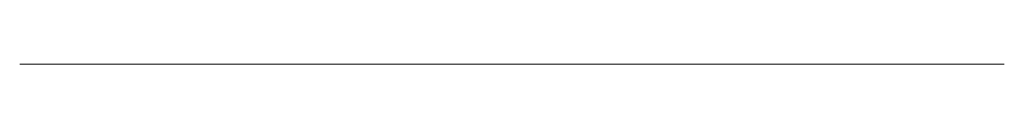
# Model space of a CAD drawing. Units: millimetres. Extents: x 1021 to 1156, y 0 to 0.
import ezdxf

# ---------------------------------------------------------------- set-up
doc = ezdxf.new("R2010")
doc.units = ezdxf.units.MM
doc.layers.add('M-CONS', color=8, linetype='Continuous', lineweight=18)

msp = doc.modelspace()

# ---------------------------------------------------------------- linework, layer by layer
at = {"layer": 'M-CONS', "extrusion": (0, -1, 0)}
for points in [[(1020.87, 534.81), (1036.46, 534.81, -1), (1036.46, 516.81), (1020.87, 516.81, 3.732051)], [(1097.93, 514.25, -0.291696), (1075.54, 517.23, 1.112381), (1063.31, 499.09, 0.317643), (1104.52, 504.39, 0.856933)]]:
    msp.add_lwpolyline(points, format="xyb", close=True, dxfattribs=at)
for points in [[(1036.46, 543.81), (1093.46, 543.81, -0.367894), (1107.28, 532.05, 0.367894), (1118.14, 522.81), (1142.46, 522.81)], [(1142.46, 494.81), (1096.42, 494.81, 0.704113), (1091.34, 480.63)]]:
    msp.add_lwpolyline(points, format="xyb", dxfattribs=at)
for centre, radius in [((1082.46, 469.81), 14), ((1082.46, 469.81), 7), ((1093.46, 529.81), 7), ((1142.46, 508.81), 14), ((1142.46, 508.81), 7)]:
    msp.add_circle(centre, radius, dxfattribs=at)
msp.add_arc((1020.1, 460.84), 49, 8.1879, 75.8686, dxfattribs=at)

doc.saveas('drawing.dxf')
